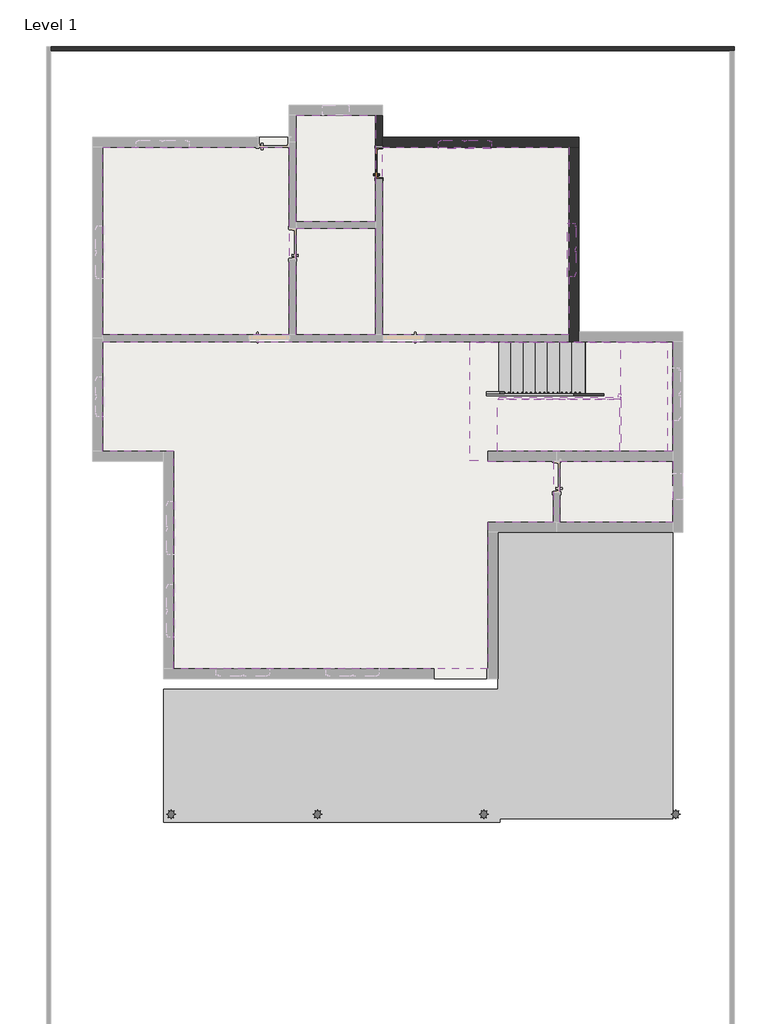
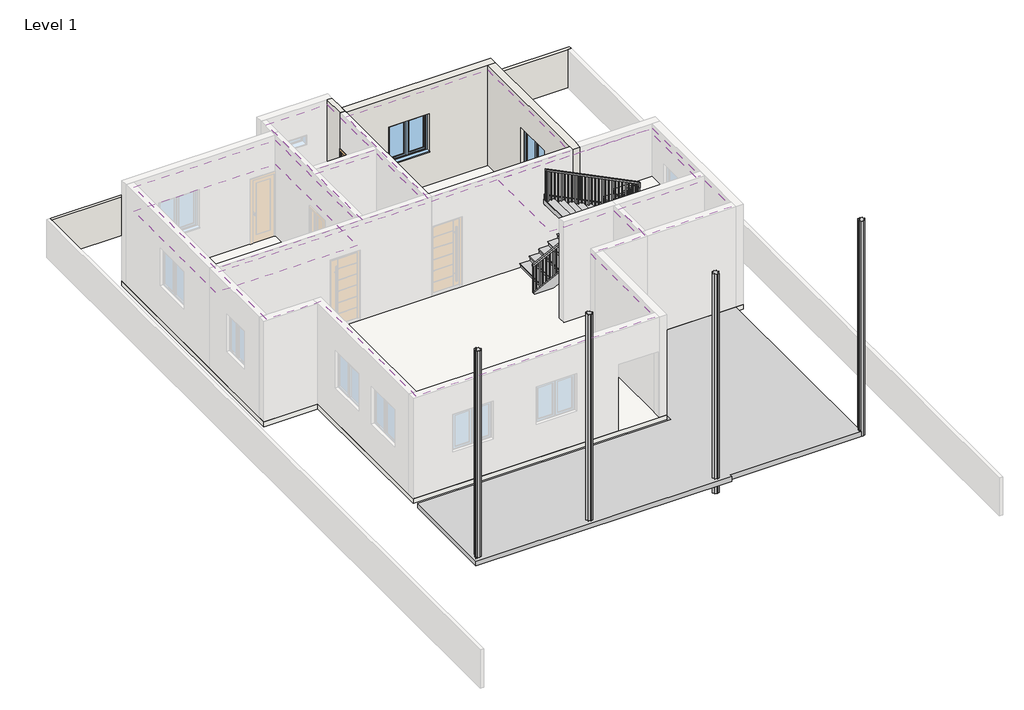
# One storey, part 2 of 2: 7 coverings, 4 walls, 3 members, 2 proxies, 2 slabs, 2 stair flights, 2 windows, 1 door, 1 railing.
"""IFC4 building model written with IfcOpenShell, lengths in millimetres."""

from ifc_helpers import new_model, si_unit, frame, origin, origin_with_axes, place, context, project, spatial, polyline, outline, extrude, faceted_brep, transform, mapped, element, save
from components import generic_models_1_generic_models_1_27fef2d6, generic_models_3_generic_models_3_d497b559, door_69f71937, non_monolithic_landing_1be43128, stair_flight_1a668dfb, stair_flight_799f9057, awning_casement_double_4_37d249be

model = new_model("IFC4")

# Units and contexts
model_context = context("Model", 3, world=origin())
ifc_project = project(units=[si_unit("LENGTHUNIT", "METRE", prefix="MILLI")], contexts=[model_context])

# Site, building, storey
site = spatial("IfcSite", under=ifc_project)
building = spatial("IfcBuilding", under=site)
storey = spatial("IfcBuildingStorey", under=building, Name="Level 1", Elevation=0.0)

# Proxies
placement = place(None, origin())
generic_models_1_generic_models_1_shape = generic_models_1_generic_models_1_27fef2d6(model_context)
element("IfcBuildingElementProxy", 1, Name="Generic Models 1 : Generic Models 1", ObjectType="Generic Models 1 : Generic Models 1", at=placement, inside=storey, context=model_context, shape_type="MappedRepresentation", body=[
    mapped(generic_models_1_generic_models_1_shape, transform((0.0, 0.0, 0.0), x_axis=(1.0, 0.0, 0.0), y_axis=(0.0, 1.0, 0.0), z_axis=(0.0, 0.0, 1.0))),
])
generic_models_3_generic_models_3_shape = generic_models_3_generic_models_3_d497b559(model_context)
element("IfcBuildingElementProxy", 2, Name="Generic Models 3 : Generic Models 3", ObjectType="Generic Models 3 : Generic Models 3", at=placement, inside=storey, context=model_context, shape_type="MappedRepresentation", body=[
    mapped(generic_models_3_generic_models_3_shape, transform((0.0, 0.0, 0.0), x_axis=(1.0, 0.0, 0.0), y_axis=(0.0, 1.0, 0.0), z_axis=(0.0, 0.0, 1.0))),
])

# Coverings
element("IfcCovering", 3, ObjectType="2' x 4' ACT System", at=placement, inside=storey, context=model_context, shape_type="SweptSolid", body=[
    extrude(outline(polyline([(-21725.4535712, 7806.8393562), (-17458.2535712, 7806.8393562), (-17458.2535712, 3514.2393562), (-21725.4535712, 3514.2393562), (-21725.4535712, 7806.8393562)])), frame((0.0, 0.0, 2438.4), z_axis=(0.0, 0.0, 1.0), x_axis=(1.0, 0.0, 0.0)), (0.0, 0.0, 1.0), 57.15),
])
element("IfcCovering", 4, ObjectType="2' x 4' ACT System", at=placement, inside=storey, context=model_context, shape_type="SweptSolid", body=[
    extrude(outline(polyline([(-21725.4535712, 7806.8393562), (-17458.2535712, 7806.8393562), (-17458.2535712, 3514.2393562), (-21725.4535712, 3514.2393562), (-21725.4535712, 7806.8393562)])), frame((0.0, 0.0, 3200.4), z_axis=(0.0, 0.0, 1.0), x_axis=(1.0, 0.0, 0.0)), (0.0, 0.0, 1.0), 57.15),
])
element("IfcCovering", 5, ObjectType="2' x 4' ACT System", at=placement, inside=storey, context=model_context, shape_type="SweptSolid", body=[
    extrude(outline(polyline([(-17305.8535712, 8543.4393562), (-15477.0535712, 8543.4393562), (-15477.0535712, 7844.9393562), (-15477.0535712, 6105.0393562), (-17305.8535712, 6105.0393562), (-17305.8535712, 7946.5393562), (-17305.8535712, 8543.4393562)])), frame((0.0, 0.0, 3200.4), z_axis=(0.0, 0.0, 1.0), x_axis=(1.0, 0.0, 0.0)), (0.0, 0.0, 1.0), 57.15),
])
element("IfcCovering", 6, ObjectType="2' x 4' ACT System", at=placement, inside=storey, context=model_context, shape_type="SweptSolid", body=[
    extrude(outline(polyline([(-17305.8535712, 3514.2393562), (-17305.8535712, 5952.6393562), (-15477.0535712, 5952.6393562), (-15477.0535712, 3514.2393562), (-17305.8535712, 3514.2393562)])), frame((0.0, 0.0, 3200.4), z_axis=(0.0, 0.0, 1.0), x_axis=(1.0, 0.0, 0.0)), (0.0, 0.0, 1.0), 57.15),
])
element("IfcCovering", 7, ObjectType="2' x 4' ACT System", at=placement, inside=storey, context=model_context, shape_type="SweptSolid", body=[
    extrude(outline(polyline([(-15324.6535712, 3514.2393562), (-15324.6535712, 7806.8393562), (-11057.4535712, 7806.8393562), (-11057.4535712, 3514.2393562), (-15324.6535712, 3514.2393562)])), frame((0.0, 0.0, 3200.4), z_axis=(0.0, 0.0, 1.0), x_axis=(1.0, 0.0, 0.0)), (0.0, 0.0, 1.0), 57.15),
])
element("IfcCovering", 8, ObjectType="2' x 4' ACT System", at=placement, inside=storey, context=model_context, shape_type="SweptSolid", body=[
    extrude(outline(polyline([(-21725.4535712, 3361.8393562), (-15311.9535712, 3361.8393562), (-10943.1535712, 3361.8393562), (-8669.8535712, 3361.8393562), (-8669.8535712, 847.2393562), (-8791.0183666, 847.2393562), (-8791.0183666, 3332.9503619), (-13326.4629678, 3332.9503619), (-13326.4629678, 640.5503619), (-12911.6535712, 640.5503619), (-12911.6535712, 618.6393562), (-11413.0535712, 618.6393562), (-11413.0535712, -778.3606438), (-12911.6535712, -778.3606438), (-12911.6535712, -4131.1606438), (-20099.8535712, -4131.1606438), (-20099.8535712, 847.2393562), (-21725.4535712, 847.2393562), (-21725.4535712, 3361.8393562)])), frame((0.0, 0.0, 3200.4), z_axis=(0.0, 0.0, 1.0), x_axis=(1.0, 0.0, 0.0)), (0.0, 0.0, 1.0), 57.15),
])
element("IfcCovering", 9, ObjectType="2' x 4' ACT System", at=placement, inside=storey, context=model_context, shape_type="SweptSolid", body=[
    extrude(outline(polyline([(-8669.8535712, 618.6393562), (-8669.8535712, -778.3606438), (-11260.6535712, -778.3606438), (-11260.6535712, 618.6393562), (-8669.8535712, 618.6393562)])), frame((0.0, 0.0, 3200.4), z_axis=(0.0, 0.0, 1.0), x_axis=(1.0, 0.0, 0.0)), (0.0, 0.0, 1.0), 57.15),
])

# Door
door_shape = door_69f71937(model_context)
element("IfcDoor", 10, ObjectType="M_Door-Interior-Single-1_Panel-Wood : 2'2\"", at=placement, inside=storey, context=model_context, shape_type="MappedRepresentation", body=[
    mapped(door_shape, transform((-15404.0285712, 7444.8893562, 152.4), x_axis=(0.0, 1.0, 0.0), y_axis=(-1.0, 0.0, 0.0), z_axis=(0.0, 0.0, 1.0))),
])

# Members
element("IfcMember", 11, ObjectType="Stringer - 2\" Width", at=placement, inside=storey, context=model_context, shape_type="SweptSolid", body=[
    extrude(outline(polyline([(202.9564199, -12936.8532683), (0.0, -12936.8532683), (0.0, -12660.658836), (1367.7751048, -9914.2532683), (1708.2829021, -9914.2532683), (202.9564199, -12936.8532683)])), frame((0.0, 2117.2393562, 0.0), z_axis=(0.0, 1.0, 0.0), x_axis=(0.0, 0.0, 1.0)), (0.0, 0.0, 1.0), 50.8),
])
element("IfcMember", 12, ObjectType="Stringer - 2\" Width", at=placement, inside=storey, context=model_context, shape_type="SweptSolid", body=[
    extrude(outline(polyline([(1532.2225356, -9863.4532683), (1872.7303329, -9863.4532683), (3264.2085938, -12657.4532683), (2923.7007965, -12657.4532683), (1532.2225356, -9863.4532683)])), frame((0.0, 2041.0393562, 0.0), z_axis=(0.0, 1.0, 0.0), x_axis=(0.0, 0.0, 1.0)), (0.0, 0.0, 1.0), 50.8),
])
element("IfcMember", 13, ObjectType="Stringer - 2\" Width", at=placement, inside=storey, context=model_context, shape_type="SweptSolid", body=[
    extrude(outline(polyline([(-9914.2532683, 2168.0393562), (-9863.4532683, 2168.0393562), (-9863.4532683, 2091.8393562), (-9914.2532683, 2091.8393562), (-9914.2532683, 2168.0393562)])), frame((0.0, 0.0, 1441.173913), z_axis=(0.0, 0.0, 1.0), x_axis=(1.0, 0.0, 0.0)), (0.0, 0.0, 1.0), 304.8),
])

# Railing
element("IfcRailing", 14, ObjectType="Handrail - Rectangular", at=placement, inside=storey, context=model_context, shape_type="SolidModel", body=[
    faceted_brep([(-12936.8532683, 2218.8393562, 1053.5478261), (-12936.8532683, 2218.8393562, 996.7965265), (-12936.8532683, 2168.0393562, 996.7965265), (-12936.8532683, 2168.0393562, 1053.5478261), (-9939.6532683, 2218.8393562, 2546.2245059), (-9888.8532683, 2218.8393562, 2514.7728111), (-9888.8532683, 2168.0393562, 2514.7728111), (-9939.6532683, 2168.0393562, 2546.2245059), (-9939.6532683, 2218.8393562, 2584.173913), (-9888.8532683, 2218.8393562, 2533.373913), (-9888.8532683, 2168.0393562, 2533.373913), (-9939.6532683, 2168.0393562, 2584.173913), (-9812.6532683, 2218.8393562, 2584.173913), (-9812.6532683, 2218.8393562, 2533.373913), (-9863.4532683, 2168.0393562, 2533.373913), (-9863.4532683, 2168.0393562, 2584.173913), (-9812.6532683, 2091.8393562, 2584.173913), (-9812.6532683, 2091.8393562, 2533.373913), (-9863.4532683, 2091.8393562, 2533.373913), (-9863.4532683, 2091.8393562, 2584.173913), (-9812.6532683, 2041.0393562, 2584.173913), (-9863.4532683, 2041.0393562, 2584.173913), (-9863.4532683, 1990.2393562, 2533.373913), (-9812.6532683, 1990.2393562, 2533.373913)], [[[0, 1, 2, 3]], [[1, 0, 4, 5]], [[2, 1, 5, 6]], [[3, 2, 6, 7]], [[0, 3, 7, 4]], [[5, 4, 8, 9]], [[6, 5, 9, 10]], [[7, 6, 10, 11]], [[4, 7, 11, 8]], [[9, 8, 12, 13]], [[10, 9, 13, 14]], [[11, 10, 14, 15]], [[8, 11, 15, 12]], [[13, 12, 16, 17]], [[14, 13, 17, 18]], [[15, 14, 18, 19]], [[12, 15, 19, 16]], [[20, 21, 22, 23]], [[17, 16, 20, 23]], [[18, 17, 23, 22]], [[19, 18, 22, 21]], [[16, 19, 21, 20]]]),
    faceted_brep([(-9812.6532683, 2041.0393562, 2584.173913), (-9812.6532683, 1990.2393562, 2533.373913), (-9863.4532683, 1990.2393562, 2533.373913), (-9863.4532683, 2041.0393562, 2584.173913), (-9812.6532683, 2041.0393562, 2698.0221344), (-9863.4532683, 2041.0393562, 2666.5704396), (-9863.4532683, 1990.2393562, 2666.5704396), (-9812.6532683, 1990.2393562, 2698.0221344)], [[[0, 1, 2, 3]], [[4, 5, 6, 7]], [[1, 0, 4, 7]], [[2, 1, 7, 6]], [[3, 2, 6, 5]], [[0, 3, 5, 4]]]),
    faceted_brep([(-9812.6532683, 1990.2393562, 2698.0221344), (-9863.4532683, 1990.2393562, 2666.5704396), (-9863.4532683, 2041.0393562, 2666.5704396), (-9812.6532683, 2041.0393562, 2698.0221344), (-12657.4532683, 1990.2393562, 4114.8), (-12657.4532683, 2041.0393562, 4114.8), (-12657.4532683, 2041.0393562, 4058.0487005), (-12657.4532683, 1990.2393562, 4058.0487005)], [[[0, 1, 2, 3]], [[4, 5, 6, 7]], [[1, 0, 4, 7]], [[2, 1, 7, 6]], [[3, 2, 6, 5]], [[0, 3, 5, 4]]]),
    extrude(outline(polyline([(4015.3556175, -12571.7282683), (4024.8429692, -12590.7782683), (3061.2521739, -12590.7782683), (3061.2521739, -12571.7282683), (4015.3556175, -12571.7282683)])), frame((0.0, 2006.1143562, 0.0), z_axis=(0.0, 1.0, 0.0), x_axis=(0.0, 0.0, 1.0)), (0.0, 0.0, 1.0), 19.05),
    extrude(outline(polyline([(3964.756408, -12470.1282683), (3974.2437597, -12489.1782683), (3061.2521739, -12489.1782683), (3061.2521739, -12470.1282683), (3964.756408, -12470.1282683)])), frame((0.0, 2006.1143562, 0.0), z_axis=(0.0, 1.0, 0.0), x_axis=(0.0, 0.0, 1.0)), (0.0, 0.0, 1.0), 19.05),
    extrude(outline(polyline([(3914.1571985, -12368.5282683), (3923.6445503, -12387.5782683), (3061.2521739, -12387.5782683), (3061.2521739, -12368.5282683), (3914.1571985, -12368.5282683)])), frame((0.0, 2006.1143562, 0.0), z_axis=(0.0, 1.0, 0.0), x_axis=(0.0, 0.0, 1.0)), (0.0, 0.0, 1.0), 19.05),
    extrude(outline(polyline([(3863.557989, -12266.9282683), (3873.0453408, -12285.9782683), (2922.1043478, -12285.9782683), (2922.1043478, -12266.9282683), (3863.557989, -12266.9282683)])), frame((0.0, 2006.1143562, 0.0), z_axis=(0.0, 1.0, 0.0), x_axis=(0.0, 0.0, 1.0)), (0.0, 0.0, 1.0), 19.05),
    extrude(outline(polyline([(3812.9587795, -12165.3282683), (3822.4461313, -12184.3782683), (2922.1043478, -12184.3782683), (2922.1043478, -12165.3282683), (3812.9587795, -12165.3282683)])), frame((0.0, 2006.1143562, 0.0), z_axis=(0.0, 1.0, 0.0), x_axis=(0.0, 0.0, 1.0)), (0.0, 0.0, 1.0), 19.05),
    extrude(outline(polyline([(3762.35957, -12063.7282683), (3771.8469218, -12082.7782683), (2782.9565217, -12082.7782683), (2782.9565217, -12063.7282683), (3762.35957, -12063.7282683)])), frame((0.0, 2006.1143562, 0.0), z_axis=(0.0, 1.0, 0.0), x_axis=(0.0, 0.0, 1.0)), (0.0, 0.0, 1.0), 19.05),
    extrude(outline(polyline([(3711.7603605, -11962.1282683), (3721.2477123, -11981.1782683), (2782.9565217, -11981.1782683), (2782.9565217, -11962.1282683), (3711.7603605, -11962.1282683)])), frame((0.0, 2006.1143562, 0.0), z_axis=(0.0, 1.0, 0.0), x_axis=(0.0, 0.0, 1.0)), (0.0, 0.0, 1.0), 19.05),
    extrude(outline(polyline([(3661.161151, -11860.5282683), (3670.6485028, -11879.5782683), (2782.9565217, -11879.5782683), (2782.9565217, -11860.5282683), (3661.161151, -11860.5282683)])), frame((0.0, 2006.1143562, 0.0), z_axis=(0.0, 1.0, 0.0), x_axis=(0.0, 0.0, 1.0)), (0.0, 0.0, 1.0), 19.05),
    extrude(outline(polyline([(3610.5619416, -11758.9282683), (3620.0492933, -11777.9782683), (2643.8086957, -11777.9782683), (2643.8086957, -11758.9282683), (3610.5619416, -11758.9282683)])), frame((0.0, 2006.1143562, 0.0), z_axis=(0.0, 1.0, 0.0), x_axis=(0.0, 0.0, 1.0)), (0.0, 0.0, 1.0), 19.05),
    extrude(outline(polyline([(3559.9627321, -11657.3282683), (3569.4500839, -11676.3782683), (2643.8086957, -11676.3782683), (2643.8086957, -11657.3282683), (3559.9627321, -11657.3282683)])), frame((0.0, 2006.1143562, 0.0), z_axis=(0.0, 1.0, 0.0), x_axis=(0.0, 0.0, 1.0)), (0.0, 0.0, 1.0), 19.05),
    extrude(outline(polyline([(3509.3635226, -11555.7282683), (3518.8508744, -11574.7782683), (2643.8086957, -11574.7782683), (2643.8086957, -11555.7282683), (3509.3635226, -11555.7282683)])), frame((0.0, 2006.1143562, 0.0), z_axis=(0.0, 1.0, 0.0), x_axis=(0.0, 0.0, 1.0)), (0.0, 0.0, 1.0), 19.05),
    extrude(outline(polyline([(3458.7643131, -11454.1282683), (3468.2516649, -11473.1782683), (2504.6608696, -11473.1782683), (2504.6608696, -11454.1282683), (3458.7643131, -11454.1282683)])), frame((0.0, 2006.1143562, 0.0), z_axis=(0.0, 1.0, 0.0), x_axis=(0.0, 0.0, 1.0)), (0.0, 0.0, 1.0), 19.05),
    extrude(outline(polyline([(3408.1651036, -11352.5282683), (3417.6524554, -11371.5782683), (2504.6608696, -11371.5782683), (2504.6608696, -11352.5282683), (3408.1651036, -11352.5282683)])), frame((0.0, 2006.1143562, 0.0), z_axis=(0.0, 1.0, 0.0), x_axis=(0.0, 0.0, 1.0)), (0.0, 0.0, 1.0), 19.05),
    extrude(outline(polyline([(3357.5658941, -11250.9282683), (3367.0532459, -11269.9782683), (2504.6608696, -11269.9782683), (2504.6608696, -11250.9282683), (3357.5658941, -11250.9282683)])), frame((0.0, 2006.1143562, 0.0), z_axis=(0.0, 1.0, 0.0), x_axis=(0.0, 0.0, 1.0)), (0.0, 0.0, 1.0), 19.05),
    extrude(outline(polyline([(3306.9666846, -11149.3282683), (3316.4540364, -11168.3782683), (2365.5130435, -11168.3782683), (2365.5130435, -11149.3282683), (3306.9666846, -11149.3282683)])), frame((0.0, 2006.1143562, 0.0), z_axis=(0.0, 1.0, 0.0), x_axis=(0.0, 0.0, 1.0)), (0.0, 0.0, 1.0), 19.05),
    extrude(outline(polyline([(3256.3674752, -11047.7282683), (3265.8548269, -11066.7782683), (2365.5130435, -11066.7782683), (2365.5130435, -11047.7282683), (3256.3674752, -11047.7282683)])), frame((0.0, 2006.1143562, 0.0), z_axis=(0.0, 1.0, 0.0), x_axis=(0.0, 0.0, 1.0)), (0.0, 0.0, 1.0), 19.05),
    extrude(outline(polyline([(3205.7682657, -10946.1282683), (3215.2556175, -10965.1782683), (2226.3652174, -10965.1782683), (2226.3652174, -10946.1282683), (3205.7682657, -10946.1282683)])), frame((0.0, 2006.1143562, 0.0), z_axis=(0.0, 1.0, 0.0), x_axis=(0.0, 0.0, 1.0)), (0.0, 0.0, 1.0), 19.05),
    extrude(outline(polyline([(3155.1690562, -10844.5282683), (3164.656408, -10863.5782683), (2226.3652174, -10863.5782683), (2226.3652174, -10844.5282683), (3155.1690562, -10844.5282683)])), frame((0.0, 2006.1143562, 0.0), z_axis=(0.0, 1.0, 0.0), x_axis=(0.0, 0.0, 1.0)), (0.0, 0.0, 1.0), 19.05),
    extrude(outline(polyline([(3104.5698467, -10742.9282683), (3114.0571985, -10761.9782683), (2226.3652174, -10761.9782683), (2226.3652174, -10742.9282683), (3104.5698467, -10742.9282683)])), frame((0.0, 2006.1143562, 0.0), z_axis=(0.0, 1.0, 0.0), x_axis=(0.0, 0.0, 1.0)), (0.0, 0.0, 1.0), 19.05),
    extrude(outline(polyline([(3053.9706372, -10641.3282683), (3063.457989, -10660.3782683), (2087.2173913, -10660.3782683), (2087.2173913, -10641.3282683), (3053.9706372, -10641.3282683)])), frame((0.0, 2006.1143562, 0.0), z_axis=(0.0, 1.0, 0.0), x_axis=(0.0, 0.0, 1.0)), (0.0, 0.0, 1.0), 19.05),
    extrude(outline(polyline([(3003.3714277, -10539.7282683), (3012.8587795, -10558.7782683), (2087.2173913, -10558.7782683), (2087.2173913, -10539.7282683), (3003.3714277, -10539.7282683)])), frame((0.0, 2006.1143562, 0.0), z_axis=(0.0, 1.0, 0.0), x_axis=(0.0, 0.0, 1.0)), (0.0, 0.0, 1.0), 19.05),
    extrude(outline(polyline([(2952.7722182, -10438.1282683), (2962.25957, -10457.1782683), (2087.2173913, -10457.1782683), (2087.2173913, -10438.1282683), (2952.7722182, -10438.1282683)])), frame((0.0, 2006.1143562, 0.0), z_axis=(0.0, 1.0, 0.0), x_axis=(0.0, 0.0, 1.0)), (0.0, 0.0, 1.0), 19.05),
    extrude(outline(polyline([(2902.1730088, -10336.5282683), (2911.6603605, -10355.5782683), (1948.0695652, -10355.5782683), (1948.0695652, -10336.5282683), (2902.1730088, -10336.5282683)])), frame((0.0, 2006.1143562, 0.0), z_axis=(0.0, 1.0, 0.0), x_axis=(0.0, 0.0, 1.0)), (0.0, 0.0, 1.0), 19.05),
    extrude(outline(polyline([(2851.5737993, -10234.9282683), (2861.061151, -10253.9782683), (1948.0695652, -10253.9782683), (1948.0695652, -10234.9282683), (2851.5737993, -10234.9282683)])), frame((0.0, 2006.1143562, 0.0), z_axis=(0.0, 1.0, 0.0), x_axis=(0.0, 0.0, 1.0)), (0.0, 0.0, 1.0), 19.05),
    extrude(outline(polyline([(2800.9745898, -10133.3282683), (2810.4619416, -10152.3782683), (1948.0695652, -10152.3782683), (1948.0695652, -10133.3282683), (2800.9745898, -10133.3282683)])), frame((0.0, 2006.1143562, 0.0), z_axis=(0.0, 1.0, 0.0), x_axis=(0.0, 0.0, 1.0)), (0.0, 0.0, 1.0), 19.05),
    extrude(outline(polyline([(2750.3753803, -10031.7282683), (2759.8627321, -10050.7782683), (1808.9217391, -10050.7782683), (1808.9217391, -10031.7282683), (2750.3753803, -10031.7282683)])), frame((0.0, 2006.1143562, 0.0), z_axis=(0.0, 1.0, 0.0), x_axis=(0.0, 0.0, 1.0)), (0.0, 0.0, 1.0), 19.05),
    extrude(outline(polyline([(2699.7761708, -9930.1282683), (2709.2635226, -9949.1782683), (1808.9217391, -9949.1782683), (1808.9217391, -9930.1282683), (2699.7761708, -9930.1282683)])), frame((0.0, 2006.1143562, 0.0), z_axis=(0.0, 1.0, 0.0), x_axis=(0.0, 0.0, 1.0)), (0.0, 0.0, 1.0), 19.05),
    extrude(outline(polyline([(-9847.5782683, 2101.3643562), (-9828.5282683, 2101.3643562), (-9828.5282683, 2082.3143562), (-9847.5782683, 2082.3143562), (-9847.5782683, 2101.3643562)])), frame((0.0, 0.0, 1669.773913), z_axis=(0.0, 0.0, 1.0), x_axis=(1.0, 0.0, 0.0)), (0.0, 0.0, 1.0), 863.6),
    extrude(outline(polyline([(-9898.3782683, 2183.9143562), (-9898.3782683, 2202.9643562), (-9879.3282683, 2202.9643562), (-9879.3282683, 2183.9143562), (-9898.3782683, 2183.9143562)])), frame((0.0, 0.0, 1530.626087), z_axis=(0.0, 0.0, 1.0), x_axis=(1.0, 0.0, 0.0)), (0.0, 0.0, 1.0), 1002.7478261),
    extrude(outline(polyline([(2468.9172775, -9980.9282683), (2459.4299258, -9999.9782683), (1530.626087, -9999.9782683), (1530.626087, -9980.9282683), (2468.9172775, -9980.9282683)])), frame((0.0, 2183.9143562, 0.0), z_axis=(0.0, 1.0, 0.0), x_axis=(0.0, 0.0, 1.0)), (0.0, 0.0, 1.0), 19.05),
    extrude(outline(polyline([(2418.318068, -10082.5282683), (2408.8307163, -10101.5782683), (1530.626087, -10101.5782683), (1530.626087, -10082.5282683), (2418.318068, -10082.5282683)])), frame((0.0, 2183.9143562, 0.0), z_axis=(0.0, 1.0, 0.0), x_axis=(0.0, 0.0, 1.0)), (0.0, 0.0, 1.0), 19.05),
    extrude(outline(polyline([(2367.7188586, -10184.1282683), (2358.2315068, -10203.1782683), (1391.4782609, -10203.1782683), (1391.4782609, -10184.1282683), (2367.7188586, -10184.1282683)])), frame((0.0, 2183.9143562, 0.0), z_axis=(0.0, 1.0, 0.0), x_axis=(0.0, 0.0, 1.0)), (0.0, 0.0, 1.0), 19.05),
    extrude(outline(polyline([(2317.1196491, -10285.7282683), (2307.6322973, -10304.7782683), (1391.4782609, -10304.7782683), (1391.4782609, -10285.7282683), (2317.1196491, -10285.7282683)])), frame((0.0, 2183.9143562, 0.0), z_axis=(0.0, 1.0, 0.0), x_axis=(0.0, 0.0, 1.0)), (0.0, 0.0, 1.0), 19.05),
    extrude(outline(polyline([(2266.5204396, -10387.3282683), (2257.0330878, -10406.3782683), (1391.4782609, -10406.3782683), (1391.4782609, -10387.3282683), (2266.5204396, -10387.3282683)])), frame((0.0, 2183.9143562, 0.0), z_axis=(0.0, 1.0, 0.0), x_axis=(0.0, 0.0, 1.0)), (0.0, 0.0, 1.0), 19.05),
    extrude(outline(polyline([(2215.9212301, -10488.9282683), (2206.4338783, -10507.9782683), (1252.3304348, -10507.9782683), (1252.3304348, -10488.9282683), (2215.9212301, -10488.9282683)])), frame((0.0, 2183.9143562, 0.0), z_axis=(0.0, 1.0, 0.0), x_axis=(0.0, 0.0, 1.0)), (0.0, 0.0, 1.0), 19.05),
    extrude(outline(polyline([(2165.3220206, -10590.5282683), (2155.8346688, -10609.5782683), (1252.3304348, -10609.5782683), (1252.3304348, -10590.5282683), (2165.3220206, -10590.5282683)])), frame((0.0, 2183.9143562, 0.0), z_axis=(0.0, 1.0, 0.0), x_axis=(0.0, 0.0, 1.0)), (0.0, 0.0, 1.0), 19.05),
    extrude(outline(polyline([(2114.7228111, -10692.1282683), (2105.2354593, -10711.1782683), (1252.3304348, -10711.1782683), (1252.3304348, -10692.1282683), (2114.7228111, -10692.1282683)])), frame((0.0, 2183.9143562, 0.0), z_axis=(0.0, 1.0, 0.0), x_axis=(0.0, 0.0, 1.0)), (0.0, 0.0, 1.0), 19.05),
    extrude(outline(polyline([(2064.1236016, -10793.7282683), (2054.6362499, -10812.7782683), (1113.1826087, -10812.7782683), (1113.1826087, -10793.7282683), (2064.1236016, -10793.7282683)])), frame((0.0, 2183.9143562, 0.0), z_axis=(0.0, 1.0, 0.0), x_axis=(0.0, 0.0, 1.0)), (0.0, 0.0, 1.0), 19.05),
    extrude(outline(polyline([(2013.5243922, -10895.3282683), (2004.0370404, -10914.3782683), (1113.1826087, -10914.3782683), (1113.1826087, -10895.3282683), (2013.5243922, -10895.3282683)])), frame((0.0, 2183.9143562, 0.0), z_axis=(0.0, 1.0, 0.0), x_axis=(0.0, 0.0, 1.0)), (0.0, 0.0, 1.0), 19.05),
    extrude(outline(polyline([(1962.9251827, -10996.9282683), (1953.4378309, -11015.9782683), (974.0347826, -11015.9782683), (974.0347826, -10996.9282683), (1962.9251827, -10996.9282683)])), frame((0.0, 2183.9143562, 0.0), z_axis=(0.0, 1.0, 0.0), x_axis=(0.0, 0.0, 1.0)), (0.0, 0.0, 1.0), 19.05),
    extrude(outline(polyline([(1912.3259732, -11098.5282683), (1902.8386214, -11117.5782683), (974.0347826, -11117.5782683), (974.0347826, -11098.5282683), (1912.3259732, -11098.5282683)])), frame((0.0, 2183.9143562, 0.0), z_axis=(0.0, 1.0, 0.0), x_axis=(0.0, 0.0, 1.0)), (0.0, 0.0, 1.0), 19.05),
    extrude(outline(polyline([(1861.7267637, -11200.1282683), (1852.2394119, -11219.1782683), (974.0347826, -11219.1782683), (974.0347826, -11200.1282683), (1861.7267637, -11200.1282683)])), frame((0.0, 2183.9143562, 0.0), z_axis=(0.0, 1.0, 0.0), x_axis=(0.0, 0.0, 1.0)), (0.0, 0.0, 1.0), 19.05),
    extrude(outline(polyline([(1811.1275542, -11301.7282683), (1801.6402024, -11320.7782683), (834.8869565, -11320.7782683), (834.8869565, -11301.7282683), (1811.1275542, -11301.7282683)])), frame((0.0, 2183.9143562, 0.0), z_axis=(0.0, 1.0, 0.0), x_axis=(0.0, 0.0, 1.0)), (0.0, 0.0, 1.0), 19.05),
    extrude(outline(polyline([(1760.5283447, -11403.3282683), (1751.0409929, -11422.3782683), (834.8869565, -11422.3782683), (834.8869565, -11403.3282683), (1760.5283447, -11403.3282683)])), frame((0.0, 2183.9143562, 0.0), z_axis=(0.0, 1.0, 0.0), x_axis=(0.0, 0.0, 1.0)), (0.0, 0.0, 1.0), 19.05),
    extrude(outline(polyline([(1709.9291352, -11504.9282683), (1700.4417835, -11523.9782683), (834.8869565, -11523.9782683), (834.8869565, -11504.9282683), (1709.9291352, -11504.9282683)])), frame((0.0, 2183.9143562, 0.0), z_axis=(0.0, 1.0, 0.0), x_axis=(0.0, 0.0, 1.0)), (0.0, 0.0, 1.0), 19.05),
    extrude(outline(polyline([(1659.3299258, -11606.5282683), (1649.842574, -11625.5782683), (695.7391304, -11625.5782683), (695.7391304, -11606.5282683), (1659.3299258, -11606.5282683)])), frame((0.0, 2183.9143562, 0.0), z_axis=(0.0, 1.0, 0.0), x_axis=(0.0, 0.0, 1.0)), (0.0, 0.0, 1.0), 19.05),
    extrude(outline(polyline([(1608.7307163, -11708.1282683), (1599.2433645, -11727.1782683), (695.7391304, -11727.1782683), (695.7391304, -11708.1282683), (1608.7307163, -11708.1282683)])), frame((0.0, 2183.9143562, 0.0), z_axis=(0.0, 1.0, 0.0), x_axis=(0.0, 0.0, 1.0)), (0.0, 0.0, 1.0), 19.05),
    extrude(outline(polyline([(1558.1315068, -11809.7282683), (1548.644155, -11828.7782683), (695.7391304, -11828.7782683), (695.7391304, -11809.7282683), (1558.1315068, -11809.7282683)])), frame((0.0, 2183.9143562, 0.0), z_axis=(0.0, 1.0, 0.0), x_axis=(0.0, 0.0, 1.0)), (0.0, 0.0, 1.0), 19.05),
    extrude(outline(polyline([(1507.5322973, -11911.3282683), (1498.0449455, -11930.3782683), (556.5913043, -11930.3782683), (556.5913043, -11911.3282683), (1507.5322973, -11911.3282683)])), frame((0.0, 2183.9143562, 0.0), z_axis=(0.0, 1.0, 0.0), x_axis=(0.0, 0.0, 1.0)), (0.0, 0.0, 1.0), 19.05),
    extrude(outline(polyline([(1456.9330878, -12012.9282683), (1447.445736, -12031.9782683), (556.5913043, -12031.9782683), (556.5913043, -12012.9282683), (1456.9330878, -12012.9282683)])), frame((0.0, 2183.9143562, 0.0), z_axis=(0.0, 1.0, 0.0), x_axis=(0.0, 0.0, 1.0)), (0.0, 0.0, 1.0), 19.05),
    extrude(outline(polyline([(1406.3338783, -12114.5282683), (1396.8465265, -12133.5782683), (417.4434783, -12133.5782683), (417.4434783, -12114.5282683), (1406.3338783, -12114.5282683)])), frame((0.0, 2183.9143562, 0.0), z_axis=(0.0, 1.0, 0.0), x_axis=(0.0, 0.0, 1.0)), (0.0, 0.0, 1.0), 19.05),
    extrude(outline(polyline([(1355.7346688, -12216.1282683), (1346.2473171, -12235.1782683), (417.4434783, -12235.1782683), (417.4434783, -12216.1282683), (1355.7346688, -12216.1282683)])), frame((0.0, 2183.9143562, 0.0), z_axis=(0.0, 1.0, 0.0), x_axis=(0.0, 0.0, 1.0)), (0.0, 0.0, 1.0), 19.05),
    extrude(outline(polyline([(1305.1354593, -12317.7282683), (1295.6481076, -12336.7782683), (417.4434783, -12336.7782683), (417.4434783, -12317.7282683), (1305.1354593, -12317.7282683)])), frame((0.0, 2183.9143562, 0.0), z_axis=(0.0, 1.0, 0.0), x_axis=(0.0, 0.0, 1.0)), (0.0, 0.0, 1.0), 19.05),
    extrude(outline(polyline([(1254.5362499, -12419.3282683), (1245.0488981, -12438.3782683), (278.2956522, -12438.3782683), (278.2956522, -12419.3282683), (1254.5362499, -12419.3282683)])), frame((0.0, 2183.9143562, 0.0), z_axis=(0.0, 1.0, 0.0), x_axis=(0.0, 0.0, 1.0)), (0.0, 0.0, 1.0), 19.05),
    extrude(outline(polyline([(1203.9370404, -12520.9282683), (1194.4496886, -12539.9782683), (278.2956522, -12539.9782683), (278.2956522, -12520.9282683), (1203.9370404, -12520.9282683)])), frame((0.0, 2183.9143562, 0.0), z_axis=(0.0, 1.0, 0.0), x_axis=(0.0, 0.0, 1.0)), (0.0, 0.0, 1.0), 19.05),
    extrude(outline(polyline([(1153.3378309, -12622.5282683), (1143.8504791, -12641.5782683), (278.2956522, -12641.5782683), (278.2956522, -12622.5282683), (1153.3378309, -12622.5282683)])), frame((0.0, 2183.9143562, 0.0), z_axis=(0.0, 1.0, 0.0), x_axis=(0.0, 0.0, 1.0)), (0.0, 0.0, 1.0), 19.05),
    extrude(outline(polyline([(1102.7386214, -12724.1282683), (1093.2512696, -12743.1782683), (139.1478261, -12743.1782683), (139.1478261, -12724.1282683), (1102.7386214, -12724.1282683)])), frame((0.0, 2183.9143562, 0.0), z_axis=(0.0, 1.0, 0.0), x_axis=(0.0, 0.0, 1.0)), (0.0, 0.0, 1.0), 19.05),
    extrude(outline(polyline([(1052.1394119, -12825.7282683), (1042.6520601, -12844.7782683), (139.1478261, -12844.7782683), (139.1478261, -12825.7282683), (1052.1394119, -12825.7282683)])), frame((0.0, 2183.9143562, 0.0), z_axis=(0.0, 1.0, 0.0), x_axis=(0.0, 0.0, 1.0)), (0.0, 0.0, 1.0), 19.05),
    extrude(outline(polyline([(-9847.5782683, 2025.1643562), (-9828.5282683, 2025.1643562), (-9828.5282683, 2006.1143562), (-9847.5782683, 2006.1143562), (-9847.5782683, 2025.1643562)])), frame((0.0, 0.0, 1669.773913), z_axis=(0.0, 0.0, 1.0), x_axis=(1.0, 0.0, 0.0)), (0.0, 0.0, 1.0), 863.6),
    extrude(outline(polyline([(-9847.5782683, 2183.9143562), (-9847.5782683, 2202.9643562), (-9828.5282683, 2202.9643562), (-9828.5282683, 2183.9143562), (-9847.5782683, 2183.9143562)])), frame((0.0, 0.0, 1669.773913), z_axis=(0.0, 0.0, 1.0), x_axis=(1.0, 0.0, 0.0)), (0.0, 0.0, 1.0), 863.6),
    extrude(outline(polyline([(4048.5613487, -12638.4032683), (4058.0487005, -12657.4532683), (3061.2521739, -12657.4532683), (3061.2521739, -12638.4032683), (4048.5613487, -12638.4032683)])), frame((0.0, 2006.1143562, 0.0), z_axis=(0.0, 1.0, 0.0), x_axis=(0.0, 0.0, 1.0)), (0.0, 0.0, 1.0), 19.05),
    extrude(outline(polyline([(1006.2838783, -12917.8032683), (996.7965265, -12936.8532683), (139.1478261, -12936.8532683), (139.1478261, -12917.8032683), (1006.2838783, -12917.8032683)])), frame((0.0, 2183.9143562, 0.0), z_axis=(0.0, 1.0, 0.0), x_axis=(0.0, 0.0, 1.0)), (0.0, 0.0, 1.0), 19.05),
])

# Slabs
element("IfcSlab", 15, ObjectType="Generic - 6\"", at=placement, inside=storey, context=model_context, shape_type="SweptSolid", body=[
    extrude(outline(polyline([(-21954.0535712, 8035.4393562), (-17458.7447825, 8035.4393562), (-17458.7447825, 8772.0393562), (-15324.6535712, 8772.0393562), (-15324.6535712, 8035.4393562), (-10828.8535712, 8035.4393562), (-10828.8535712, 3590.4393562), (-8441.2535712, 3590.4393562), (-8441.2535712, -1006.9606438), (-12683.0535712, -1006.9606438), (-12683.0535712, -4359.7606438), (-20328.4535712, -4359.7606438), (-20328.4535712, 618.6393562), (-21954.0535712, 618.6393562), (-21954.0535712, 8035.4393562)])), origin_with_axes(), (0.0, 0.0, 1.0), 152.4),
])
non_monolithic_landing_shape = non_monolithic_landing_1be43128(model_context)
element("IfcSlab", 16, ObjectType="Non-Monolithic Landing", at=placement, inside=storey, context=model_context, shape_type="MappedRepresentation", body=[
    mapped(non_monolithic_landing_shape, transform((0.0, 0.0, 0.0), x_axis=(1.0, 0.0, 0.0), y_axis=(0.0, 1.0, 0.0), z_axis=(0.0, 0.0, 1.0))),
])

# Stair flights
stair_flight_shape = stair_flight_1a668dfb(model_context)
element("IfcStairFlight", 17, ObjectType="2\" Tread 1\" Nosing 1/4\" Riser", at=placement, inside=storey, context=model_context, shape_type="MappedRepresentation", body=[
    mapped(stair_flight_shape, transform((0.0, 0.0, 0.0), x_axis=(1.0, 0.0, 0.0), y_axis=(0.0, 1.0, 0.0), z_axis=(0.0, 0.0, 1.0))),
])
stair_flight_2_shape = stair_flight_799f9057(model_context)
element("IfcStairFlight", 18, ObjectType="2\" Tread 1\" Nosing 1/4\" Riser", at=placement, inside=storey, context=model_context, shape_type="MappedRepresentation", body=[
    mapped(stair_flight_2_shape, transform((0.0, 0.0, 0.0), x_axis=(1.0, 0.0, 0.0), y_axis=(0.0, 1.0, 0.0), z_axis=(0.0, 0.0, 1.0))),
])

# Walls
element("IfcWall", 19, ObjectType="Generic - 4\"", at=placement, inside=storey, context=model_context, shape_type="Brep", body=[
    faceted_brep([(-22914.3713098, 10013.1503619, 0.0), (-7369.5713098, 10013.1503619, 0.0), (-7267.9713098, 10013.1503619, 0.0), (-7267.9713098, 10013.1503619, 1219.2), (-7369.5713098, 10013.1503619, 1219.2), (-22914.3713098, 10013.1503619, 1219.2), (-22914.3713098, 10114.7503619, 0.0), (-22914.3713098, 10114.7503619, 1219.2), (-7267.9713098, 10114.7503619, 1219.2), (-7267.9713098, 10114.7503619, 0.0)], [[[0, 1, 2, 3, 4, 5]], [[6, 7, 8, 9]], [[2, 1, 0, 6, 9]], [[5, 4, 3, 8, 7]], [[0, 5, 7, 6]], [[3, 2, 9, 8]]]),
])
element("IfcWall", 20, ObjectType="Generic - 6\"", at=placement, inside=storey, context=model_context, shape_type="Brep", body=[
    faceted_brep([(-15477.0535712, 8543.4393562, 152.4), (-15477.0535712, 7844.9393562, 152.4), (-15477.0535712, 7844.9393562, 3352.8), (-15477.0535712, 8543.4393562, 3352.8), (-15324.6535712, 8543.4393562, 152.4), (-15324.6535712, 8543.4393562, 3352.8), (-15324.6535712, 8035.4393562, 3352.8), (-15324.6535712, 7844.9393562, 3352.8), (-15324.6535712, 7844.9393562, 152.4), (-15324.6535712, 8035.4393562, 152.4)], [[[0, 1, 2, 3]], [[4, 5, 6, 7, 8, 9]], [[1, 0, 4, 9, 8]], [[2, 1, 8, 7]], [[3, 2, 7, 6, 5]], [[0, 3, 5, 4]]]),
])
element("IfcWall", 21, ObjectType="Generic - 9\"", at=placement, inside=storey, context=model_context, shape_type="Brep", body=[
    faceted_brep([(-15324.6535712, 7806.8393562, 152.4), (-11057.4535712, 7806.8393562, 152.4), (-10828.8535712, 7806.8393562, 152.4), (-10828.8535712, 7806.8393562, 3352.8), (-11057.4535712, 7806.8393562, 3352.8), (-15324.6535712, 7806.8393562, 3352.8), (-12822.7535712, 7806.8393562, 1219.2), (-14041.9535712, 7806.8393562, 1219.2), (-14041.9535712, 7806.8393562, 2419.2), (-12822.7535712, 7806.8393562, 2419.2), (-15324.6535712, 8035.4393562, 152.4), (-15324.6535712, 8035.4393562, 3352.8), (-10828.8535712, 8035.4393562, 3352.8), (-10828.8535712, 8035.4393562, 152.4), (-12822.7535712, 8035.4393562, 1219.2), (-12822.7535712, 8035.4393562, 2419.2), (-14041.9535712, 8035.4393562, 2419.2), (-14041.9535712, 8035.4393562, 1219.2), (-15324.6535712, 7844.9393562, 152.4), (-15324.6535712, 7844.9393562, 3352.8)], [[[0, 1, 2, 3, 4, 5], [6, 7, 8, 9]], [[10, 11, 12, 13], [14, 15, 16, 17]], [[2, 1, 0, 18, 10, 13]], [[5, 4, 3, 12, 11, 19]], [[3, 2, 13, 12]], [[0, 5, 19, 11, 10, 18]], [[15, 14, 6, 9]], [[16, 15, 9, 8]], [[17, 16, 8, 7]], [[14, 17, 7, 6]]]),
])
element("IfcWall", 22, ObjectType="Generic - 9\"", at=placement, inside=storey, context=model_context, shape_type="Brep", body=[
    faceted_brep([(-11057.4535712, 7806.8393562, 152.4), (-11057.4535712, 3514.2393562, 152.4), (-11057.4535712, 3361.8393562, 152.4), (-11057.4535712, 3361.8393562, 3352.8), (-11057.4535712, 3514.2393562, 3352.8), (-11057.4535712, 7806.8393562, 3352.8), (-11057.4535712, 4847.7393562, 1219.2), (-11057.4535712, 6066.9393562, 1219.2), (-11057.4535712, 6066.9393562, 2419.2), (-11057.4535712, 4847.7393562, 2419.2), (-10828.8535712, 7806.8393562, 152.4), (-10828.8535712, 7806.8393562, 3352.8), (-10828.8535712, 3590.4393562, 3352.8), (-10828.8535712, 3361.8393562, 3352.8), (-10828.8535712, 3361.8393562, 152.4), (-10828.8535712, 3590.4393562, 152.4), (-10828.8535712, 4847.7393562, 1219.2), (-10828.8535712, 4847.7393562, 2419.2), (-10828.8535712, 6066.9393562, 2419.2), (-10828.8535712, 6066.9393562, 1219.2)], [[[0, 1, 2, 3, 4, 5], [6, 7, 8, 9]], [[10, 11, 12, 13, 14, 15], [16, 17, 18, 19]], [[2, 1, 0, 10, 15, 14]], [[5, 4, 3, 13, 12, 11]], [[0, 5, 11, 10]], [[3, 2, 14, 13]], [[17, 16, 6, 9]], [[18, 17, 9, 8]], [[19, 18, 8, 7]], [[16, 19, 7, 6]]]),
])

# Windows
awning_casement_double_4_shape = awning_casement_double_4_37d249be(model_context)
element("IfcWindow", 23, ObjectType="Awning Casement double : 4'", at=placement, inside=storey, context=model_context, shape_type="MappedRepresentation", body=[
    mapped(awning_casement_double_4_shape, transform((-13432.3535712, 7921.1393562, 419.2), x_axis=(-1.0, 0.0, 0.0), y_axis=(0.0, -1.0, 0.0), z_axis=(0.0, 0.0, 1.0))),
])
element("IfcWindow", 24, ObjectType="Awning Casement double : 4'", at=placement, inside=storey, context=model_context, shape_type="MappedRepresentation", body=[
    mapped(awning_casement_double_4_shape, transform((-10943.1535712, 5457.3393562, 419.2), x_axis=(0.0, 1.0, 0.0), y_axis=(-1.0, 0.0, 0.0), z_axis=(0.0, 0.0, 1.0))),
])

save(model, "model.ifc")

# Revit data of these elements
# Type "2' x 4' ACT System"
#   Assembly Code = "C3030210"
#   built-in parameter 1002203 = 1 (stored number, unit not read)
#   built-in parameter 1002202 = 1 (stored number, unit not read)
#   Layers, outside or top first: 0' - 1 5/8" "Default" (function 1); 0' - 0 5/8" "Acoustic Ceiling Tile 24 x 48" (function 5)
# Type "M_Door-Interior-Single-1_Panel-Wood : 2'2\""
#   Type Mark = "17"
#   Assembly Code = "C1020300"
#   Analytic Construction = "Wooden"
#   Top Rail = 0' - 4.72441"
#   Thickness = 0' - 1.37795"
#   Thermal Resistance (R) = 2.5876 (h·ft²·°F)/BTU
#   Swing Angle [instance default] = 90.00°
#   Stiles = 0' - 4.72441"
#   Rough Width = 2' - 3.9685"
#   Rough Height = 6' - 7.72441"
#   Height = 6' - 6.74016"
#   Width = 2' - 2"
#   Heat Transfer Coefficient (U) = 0.3865 BTU/(h·ft²·°F)
#   Bottom Rail = 0' - 9.05512"
#   Trim Material = Cherry
#   Panel Material = Cherry
#   Frame Material = Cherry
#   Door Handle Material = Aluminum
#   Visual Light Transmittance = 0
#   Solar Heat Gain Coefficient = 0
#   Wall Closure = (empty or 0)
#   Function = (empty or 0)
# Type "Handrail - Rectangular"
#   Assembly Code = "C2010400"
#   built-in parameter 1008612 = 0.0416667 (stored number, unit not read)
#   built-in parameter 1008611 = 0.0416667 (stored number, unit not read)
#   built-in parameter 1008609 = 0.333333 (stored number, unit not read)
#   built-in parameter 1008604 = 0.166667 (stored number, unit not read)
#   built-in parameter 1008603 = 0.166667 (stored number, unit not read)
#   Railing Height = 3' - 0"
#   built-in parameter 1008630 = 2
#   built-in parameter 1008610 = 2
#   built-in parameter 1008618 = Baluster - Square : 3/4"
# Type "Generic - 6\""
#   Assembly Code = "B1010"
#   Function = 0
#   Layers, outside or top first: 0' - 6" no material (function 1)
# Type "Generic - 4\""
#   Assembly Code = "B2010"
#   Layers, outside or top first: 0' - 4" no material (function 1)
# Type "Generic - 6\""
#   Assembly Code = "B2010"
#   Layers, outside or top first: 0' - 6" no material (function 1)
# Type "Generic - 9\""
#   Assembly Code = "B2010"
#   Layers, outside or top first: 0' - 9" no material (function 1)
# Type "Awning Casement double : 4'"
#   Type Mark = "21"
#   Operation = "DoublePanelVertical"
#   Keynote = "L10/210"
#   Height = 3' - 11.24409"
#   Default Sill Height = 2' - 7.49606"
#   Width = 4' - 0"
#   Wall Closure = (empty or 0)
# Element 1 (IfcBuildingElementProxy, "Generic Models 1 : Generic Models 1")
#   Phase Created = New Construction
# Element 2 (IfcBuildingElementProxy, "Generic Models 3 : Generic Models 3")
#   Phase Created = New Construction
#   Materials on its faces: "Acoustic Ceiling Tile 24 x 24"
# Element 3 (IfcCovering, "2' x 4' ACT System")
#   Height Offset From Level = 8' - 0"
#   Phase Created = New Construction
#   Materials on its faces: "Acoustic Ceiling Tile 24 x 48", "Default"
# Elements 4, 5, 6, 7, 8, 9 (IfcCovering, "2' x 4' ACT System")
#   Height Offset From Level = 10' - 6"
#   Phase Created = New Construction
#   Materials on its faces: "Acoustic Ceiling Tile 24 x 48", "Default"
# Element 10 (IfcDoor, "M_Door-Interior-Single-1_Panel-Wood : 2'2\"")
#   Swing Angle = 90.00°
#   Phase Created = New Construction
#   Materials on its faces: "Cherry", "Aluminum"
# Elements 11, 12, 13 (IfcMember, "Stringer - 2\" Width")
#   Phase Created = New Construction
# Element 14 (IfcRailing, "Handrail - Rectangular")
#   Phase Created = New Construction
# Element 15 (IfcSlab, "Generic - 6\"")
#   built-in parameter 1001955 = 3.14159 (stored number, unit not read)
#   Height Offset From Level = 0' - 6"
#   Phase Created = New Construction
#   Materials on its faces: "4", "Default Floor"
# Element 16 (IfcSlab, "Non-Monolithic Landing")
#   Phase Created = New Construction
# Elements 17, 18 (IfcStairFlight, "2\" Tread 1\" Nosing 1/4\" Riser")
#   Phase Created = New Construction
# Element 19 (IfcWall, "Generic - 4\"")
#   Top Offset = 0' - 0"
#   Base Offset = 0' - 0"
#   Unconnected Height = 4' - 0"
#   wall height = 4' - 0"
#   Phase Created = New Construction
#   Base Constraint = Level 1
#   Materials on its faces: "Default Wall"
# Element 20 (IfcWall, "Generic - 6\"")
#   built-in parameter 1001111 = 0' - 6"
#   Top Offset = 0' - 0"
#   Base Offset = 0' - 6"
#   Unconnected Height = 10' - 6"
#   wall height = 10' - 6"
#   Phase Created = New Construction
#   Base Constraint = Level 1
#   Materials on its faces: "Default Wall", "9"
# Element 21 (IfcWall, "Generic - 9\"")
#   built-in parameter 1001111 = 0' - 6"
#   Top Offset = 0' - 0"
#   Base Offset = 0' - 6"
#   Unconnected Height = 10' - 6"
#   wall height = 10' - 6"
#   Phase Created = New Construction
#   Base Constraint = Level 1
#   Materials on its faces: "Default Wall", "9", "2"
# Element 22 (IfcWall, "Generic - 9\"")
#   built-in parameter 1001111 = 0' - 6"
#   Top Offset = 0' - 0"
#   Base Offset = 0' - 6"
#   Unconnected Height = 10' - 6"
#   wall height = 10' - 6"
#   Phase Created = New Construction
#   Base Constraint = Level 1
#   Materials on its faces: "Default Wall", "3", "9", "7"
# Element 23 (IfcWindow, "Awning Casement double : 4'")
#   Mark = "1"
#   Phase Created = New Construction
#   Materials on its faces: "Default Frame", "Glass", "Default Sill"
# Element 24 (IfcWindow, "Awning Casement double : 4'")
#   Mark = "8"
#   Phase Created = New Construction
#   Materials on its faces: "Default Frame", "Glass", "Default Sill"
# Materials
#   "Default": colour RGB 127 127 127, transparency 0, Cost = 0
#   "Acoustic Ceiling Tile 24 x 48": class "Generic", colour RGB 229 229 229, transparency 0, Description = "Acoustic Ceiling Tile 24 x 48", Cost = 0
#   "Cherry": class "Wood", colour RGB 226 177 128, transparency 0, Description = "Prunus Serotina", Cost = 0
#   "Aluminum": class "Metal", colour RGB 247 247 247, transparency 0, Description = "Aluminum 6061", Cost = 0
#   "Acoustic Ceiling Tile 24 x 24": class "Generic", colour RGB 232 232 232, transparency 0, Description = "Acoustic Ceiling Tile 24 x 24", Cost = 0
#   "4": class "Generic", colour RGB 120 120 120, transparency 0, Cost = 0
#   "Default Floor": colour RGB 128 128 128, transparency 0, Cost = 0
#   "Default Wall": colour RGB 128 128 128, transparency 0, Cost = 0
#   "9": class "Generic", colour RGB 120 120 120, transparency 0, Cost = 0
#   "2": class "Generic", colour RGB 120 120 120, transparency 0, Cost = 0
#   "3": class "Generic", colour RGB 120 120 120, transparency 0, Cost = 0
#   "7": class "Generic", colour RGB 120 120 120, transparency 0, Cost = 0
#   "Default Frame": colour RGB 193 168 117, transparency 0
#   "Glass": class "Glass", colour RGB 0 128 192, transparency 0.75, Description = "Soda Lime Glass", Cost = 0
#   "Default Sill": colour RGB 188 165 158, transparency 0
